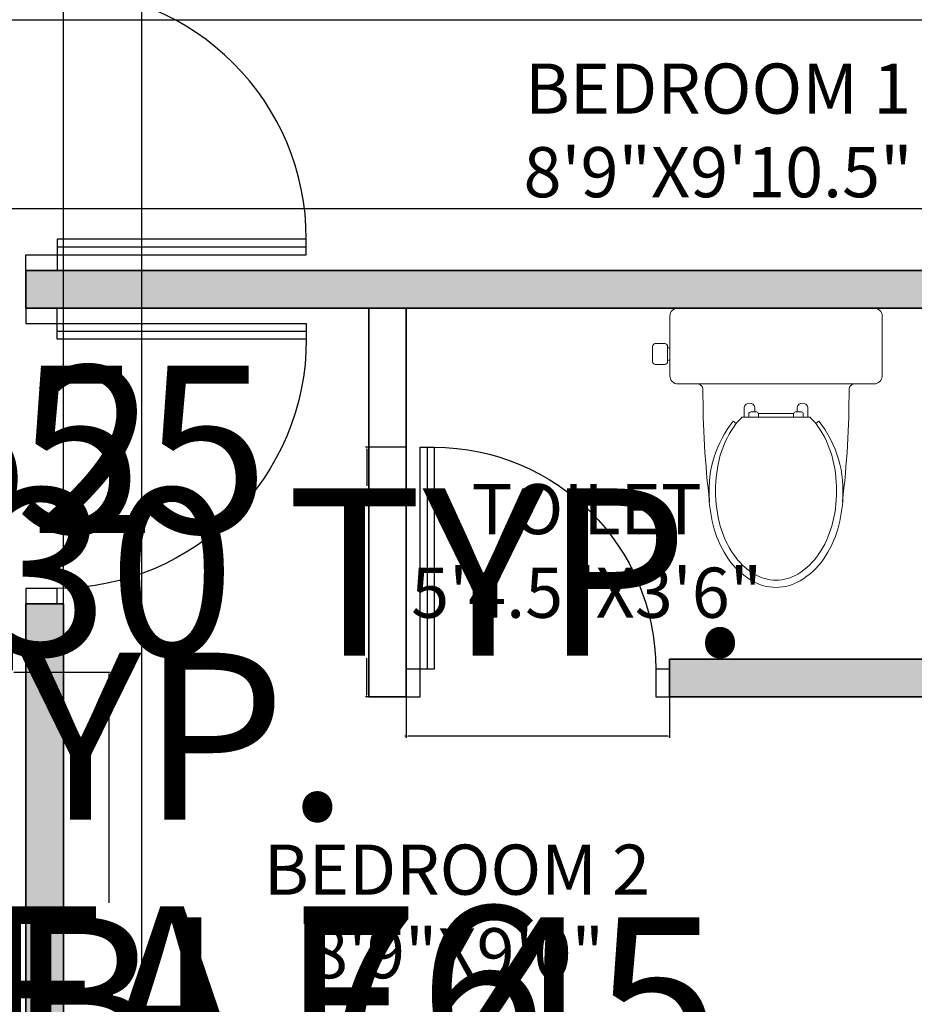
# Model space of a CAD drawing. Units: inches. Extents: x 305 to 776, y 38 to 479.
# Tile 12 of 14: x 511 to 618, y 214 to 332. Entities that reach past the tile are written whole.
import ezdxf

# ---------------------------------------------------------------- set-up
doc = ezdxf.new("R2010")
doc.units = ezdxf.units.IN
doc.header["$MEASUREMENT"] = 0
for name, color, linetype, lineweight in [('A-ANNO-DIMS', 2, 'Continuous', 18), ('A-AREA-IDEN', 7, 'Continuous', 18), ('A-DOOR', 4, 'Continuous', 25), ('A-FLOR-FIXT', 9, 'Continuous', 18), ('A-WALL', 7, 'Continuous', 35), ('A-WALL-PATT', 252, 'Continuous', 13)]:
    doc.layers.add(name, color=color, linetype=linetype, lineweight=lineweight)
doc.styles.get("Standard").update_dxf_attribs({"font": 'arial.ttf'})
doc.dimstyles.get("Standard").update_dxf_attribs({"dimtxt": 20, "dimasz": 0.18, "dimexe": 0.18, "dimexo": 0.0625, "dimgap": 0.09, "dimtad": 0, "dimtih": 1, "dimtoh": 1, "dimdec": 4, "dimzin": 0, "dimdsep": 46, "dimtxsty": 'Standard', "dimcen": 0.09, "dimadec": 0, "dimazin": 0, "dimtfac": 1, "dimtdec": 4, "dimtofl": 0, "dimtmove": 0, "dimatfit": 3, "dimfxl": 1, "dimtolj": 1, "dimtzin": 0, "dimarcsym": 0})

# ---------------------------------------------------------------- blocks, each defined once
blk = doc.blocks.new('A$C296830DC')
blk.add_line((828.9, 852.6), (828.9, 94.7))
for points in [[(852.6, 94.7), (852.6, 852.6), (805.3, 852.6), (805.3, 94.7)], [(47.4, 94.7), (47.4, 0), (0, 0), (0, 94.7)], [(900, 94.7), (900, 0), (852.6, 0), (852.6, 94.7)]]:
    blk.add_lwpolyline(points, close=True)
blk.add_arc((805.3, 94.7), 757.9, 90, 180)
blk = doc.blocks.new('t')
for points in [[(1220.28, 636.63), (1208.55, 636.63, 0.414214), (1207.58, 635.67), (1207.58, 631.86, 0.414214)], [(1220.28, 636.63), (1232.02, 636.63, -0.414214), (1232.98, 635.67), (1232.98, 628.51, -0.414214), (1232.02, 627.55), (1229.53, 627.55)], [(1207.31, 631.86), (1207.31, 632.04, 0.414214), (1206.99, 632.37), (1205.84, 632.37, 0.414214), (1205.52, 632.04), (1205.52, 630.21, 0.414214), (1205.84, 629.89)], [(1207.31, 630.39), (1207.31, 631.86, 0.414214)], [(1207.58, 631.86), (1207.58, 630.39, 0.414214)], [(1205.84, 629.89), (1206.99, 629.89, 0.414214), (1207.31, 630.21), (1207.31, 630.39, 0.414214)], [(1207.58, 630.39), (1207.58, 628.51, 0.414214), (1208.55, 627.55), (1211.03, 627.55)], [(1211.03, 627.55, -0.279901), (1211.54, 626.96, 0.030761), (1212.34, 613.45, 16.522544)], [(1229.53, 627.55, 0.279901), (1229.02, 626.96, -0.030761), (1228.22, 613.45, -16.522544)], [(1216.48, 623.56), (1216.48, 624.75, -0.788198), (1217.76, 624.75), (1217.76, 624.2)], [(1224.09, 623.56), (1224.09, 624.75, 0.788198), (1222.8, 624.75), (1222.8, 624.2)], [(1213.04, 614.76, 0.068564), (1213.62, 610.52, 0.080689), (1215.16, 607.21, 0.107047), (1217.67, 604.81, 0.137952), (1220.28, 604.08, 0.137952), (1222.89, 604.81, 0.107047), (1225.4, 607.21, 0.080689), (1226.94, 610.52, 0.068564), (1227.53, 614.76, 0.068564), (1226.94, 619.01, 0.080689), (1225.4, 622.31, 0.049741), (1224.36, 623.56, 0.137952)], [(1216.2, 623.56, 0.049741), (1215.16, 622.31, 0.080689), (1213.62, 619.01, 0.068564), (1213.04, 614.76, 0.068564)], [(1217.03, 623.56), (1217.03, 623.98, -0.414214), (1217.26, 624.2), (1217.94, 624.2, -0.414214), (1218.17, 623.98), (1218.17, 623.56)], [(1223.54, 623.56), (1223.54, 623.98, 0.414214), (1223.31, 624.2), (1222.62, 624.2, 0.414214), (1222.39, 623.98), (1222.39, 623.56)], [(1212.3, 614.03, -0.186192), (1215.17, 623.1), (1215.53, 622.81)], [(1228.22, 613.45, 0.197511), (1225.39, 623.1), (1225.04, 622.81)], [(1212.27, 614.03, 0.059006), (1212.9, 610.18, 0.081908), (1214.61, 606.59, 0.106902), (1217.38, 604.01, 0.135271), (1220.28, 603.21, 0.135271)], [(1212.34, 613.45, -0.010918), (1212.3, 614.03)], [(1220.28, 603.21, 0.135271), (1223.19, 604.01, 0.106902), (1225.95, 606.59, 0.081908), (1227.66, 610.18, 0.059006), (1228.29, 614.03, 0.070136)]]:
    blk.add_lwpolyline(points, format="xyb")
for points in [[(1207.31, 631.86), (1207.58, 631.86)], [(1207.31, 630.39), (1207.58, 630.39)], [(1211.03, 627.55), (1220.28, 627.55)], [(1229.53, 627.55), (1220.28, 627.55)], [(1216.2, 623.56), (1224.36, 623.56)], [(1218.17, 624.02), (1222.39, 624.02)]]:
    blk.add_lwpolyline(points)
blk = doc.blocks.new('*D19')
at = {"layer": 'A-ANNO-DIMS', "color": 0, "lineweight": -2, "transparency": 16777216}
for p, q in [((557.63, 250.82), (557.63, 245.98)), ((589.13, 250.82), (589.13, 245.98)), ((557.63, 246.16), (557.45, 246.16)), ((588.95, 246.16), (557.81, 246.16))]:
    blk.add_line(p, q, dxfattribs=at)
at = {"layer": 'A-ANNO-DIMS', "color": 0, "transparency": 16777216}
for points in [[(557.81, 246.19), (557.81, 246.13), (557.63, 246.16)], [(588.95, 246.19), (588.95, 246.13), (589.13, 246.16)]]:
    blk.add_solid(points, dxfattribs=at)
at = {"layer": 'Defpoints', "color": 0, "transparency": 16777216}
for p in [(557.63, 250.88), (589.13, 250.88), (557.63, 246.16)]:
    blk.add_point(p, dxfattribs=at)
at = {"layer": 'A-ANNO-DIMS', "color": 0, "transparency": 16777216, "insert": (463.39, 246.16), "char_height": 20, "attachment_point": 5}
blk.add_mtext('\\A1;DOOR 32 TYP.', dxfattribs=at)
blk = doc.blocks.new('*D20')
at = {"layer": 'A-ANNO-DIMS', "color": 0, "lineweight": -2, "transparency": 16777216}
for p, q in [((557.57, 280.72), (552.73, 280.72)), ((552.91, 280.54), (552.91, 276.11)), ((552.91, 251.06), (552.91, 255.49)), ((557.57, 250.88), (552.73, 250.88))]:
    blk.add_line(p, q, dxfattribs=at)
at = {"layer": 'A-ANNO-DIMS', "color": 0, "transparency": 16777216}
for points in [[(552.88, 280.54), (552.94, 280.54), (552.91, 280.72)], [(552.88, 251.06), (552.94, 251.06), (552.91, 250.88)]]:
    blk.add_solid(points, dxfattribs=at)
at = {"layer": 'Defpoints', "color": 0, "transparency": 16777216}
for p in [(552.91, 280.72), (557.63, 280.72), (557.63, 250.88)]:
    blk.add_point(p, dxfattribs=at)
at = {"layer": 'A-ANNO-DIMS', "color": 0, "transparency": 16777216, "insert": (552.91, 265.8), "char_height": 20, "attachment_point": 5}
blk.add_mtext('\\A1;30 TYP.', dxfattribs=at)
blk = doc.blocks.new('*D27')
at = {"layer": 'A-ANNO-DIMS', "color": 0, "lineweight": -2, "transparency": 16777216}
for p, q in [((630.7, 388.18), (639.63, 388.18)), ((639.45, 388), (639.45, 369.09)), ((639.45, 329.56), (639.45, 348.47)), ((630.7, 329.38), (639.63, 329.38))]:
    blk.add_line(p, q, dxfattribs=at)
at = {"layer": 'A-ANNO-DIMS', "color": 0, "transparency": 16777216}
for points in [[(639.42, 388), (639.48, 388), (639.45, 388.18)], [(639.42, 329.56), (639.48, 329.56), (639.45, 329.38)]]:
    blk.add_solid(points, dxfattribs=at)
at = {"layer": 'Defpoints', "color": 0, "transparency": 16777216}
for p in [(630.63, 388.18), (630.63, 329.38), (639.45, 329.38)]:
    blk.add_point(p, dxfattribs=at)
at = {"layer": 'A-ANNO-DIMS', "color": 0, "transparency": 16777216, "insert": (639.45, 358.78), "char_height": 20, "attachment_point": 5}
blk.add_mtext('\\A1;W3 59 TYP.', dxfattribs=at)
blk = doc.blocks.new('*D33')
at = {"layer": 'A-ANNO-DIMS', "color": 0, "lineweight": -2, "transparency": 16777216}
for p, q in [((440.93, 307.95), (449.29, 307.95)), ((449.11, 307.77), (449.11, 290.9)), ((449.11, 253.16), (449.11, 270.03)), ((440.93, 252.98), (449.29, 252.98))]:
    blk.add_line(p, q, dxfattribs=at)
at = {"layer": 'A-ANNO-DIMS', "color": 0, "transparency": 16777216}
for points in [[(449.08, 307.77), (449.14, 307.77), (449.11, 307.95)], [(449.08, 253.16), (449.14, 253.16), (449.11, 252.98)]]:
    blk.add_solid(points, dxfattribs=at)
at = {"layer": 'Defpoints', "color": 0, "transparency": 16777216}
for p in [(440.86, 307.95), (449.11, 307.95), (440.86, 252.98)]:
    blk.add_point(p, dxfattribs=at)
at = {"layer": 'A-ANNO-DIMS', "color": 0, "transparency": 16777216, "insert": (449.11, 280.47), "char_height": 20, "attachment_point": 5}
blk.add_mtext('\\A1;DINING SET 55', dxfattribs=at)
blk = doc.blocks.new('*D35')
at = {"layer": 'A-ANNO-DIMS', "color": 0, "lineweight": -2, "transparency": 16777216}
for p, q in [((510.7, 253.8), (522.21, 253.8)), ((522.03, 253.62), (522.03, 226.23)), ((522.03, 177.97), (522.03, 205.36)), ((510.7, 177.79), (522.21, 177.79))]:
    blk.add_line(p, q, dxfattribs=at)
at = {"layer": 'A-ANNO-DIMS', "color": 0, "transparency": 16777216}
for points in [[(522, 253.62), (522.06, 253.62), (522.03, 253.8)], [(522, 177.97), (522.06, 177.97), (522.03, 177.79)]]:
    blk.add_solid(points, dxfattribs=at)
at = {"layer": 'Defpoints', "color": 0, "transparency": 16777216}
for p in [(510.63, 253.8), (522.03, 253.8), (510.63, 177.79)]:
    blk.add_point(p, dxfattribs=at)
at = {"layer": 'A-ANNO-DIMS', "color": 0, "transparency": 16777216, "insert": (522.03, 215.8), "char_height": 20, "attachment_point": 5}
blk.add_mtext('\\A1;SOFA 76', dxfattribs=at)
blk = doc.blocks.new('*D37')
at = {"layer": 'A-ANNO-DIMS', "color": 0, "lineweight": -2, "transparency": 16777216}
for p, q in [((476.35, 237.03), (483.22, 237.03)), ((483.04, 236.85), (483.04, 224.94)), ((483.04, 192.15), (483.04, 204.06)), ((476.35, 191.97), (483.22, 191.97))]:
    blk.add_line(p, q, dxfattribs=at)
at = {"layer": 'A-ANNO-DIMS', "color": 0, "transparency": 16777216}
for points in [[(483.01, 236.85), (483.07, 236.85), (483.04, 237.03)], [(483.01, 192.15), (483.07, 192.15), (483.04, 191.97)]]:
    blk.add_solid(points, dxfattribs=at)
at = {"layer": 'Defpoints', "color": 0, "transparency": 16777216}
for p in [(476.28, 237.03), (483.04, 237.03), (476.28, 191.97)]:
    blk.add_point(p, dxfattribs=at)
at = {"layer": 'A-ANNO-DIMS', "color": 0, "transparency": 16777216, "insert": (483.04, 214.5), "char_height": 20, "attachment_point": 5}
blk.add_mtext('\\A1;COFFEE TABLE 45', dxfattribs=at)
blk = doc.blocks.new('*D49')
at = {"layer": 'A-ANNO-DIMS', "color": 0, "lineweight": -2, "transparency": 16777216}
for p, q in [((399.7, 331.88), (648.81, 331.88)), ((648.63, 331.7), (648.63, 330.88)), ((648.63, 309.46), (648.63, 310.28)), ((399.7, 309.28), (648.81, 309.28))]:
    blk.add_line(p, q, dxfattribs=at)
at = {"layer": 'A-ANNO-DIMS', "color": 0, "transparency": 16777216}
for points in [[(648.6, 331.7), (648.66, 331.7), (648.63, 331.88)], [(648.6, 309.46), (648.66, 309.46), (648.63, 309.28)]]:
    blk.add_solid(points, dxfattribs=at)
at = {"layer": 'Defpoints', "color": 0, "transparency": 16777216}
for p in [(399.63, 331.88), (648.63, 331.88), (399.63, 309.28)]:
    blk.add_point(p, dxfattribs=at)
at = {"layer": 'A-ANNO-DIMS', "color": 0, "transparency": 16777216, "insert": (648.63, 320.58), "char_height": 20, "attachment_point": 5}
blk.add_mtext('\\A1;22.6', dxfattribs=at)
blk = doc.blocks.new('*D58')
at = {"layer": 'A-ANNO-DIMS', "color": 0, "lineweight": -2, "transparency": 16777216}
for p, q in [((516.63, 138.44), (516.63, 447.56)), ((516.81, 447.38), (525.83, 447.38)), ((526.01, 138.44), (526.01, 447.56)), ((526.01, 447.38), (526.19, 447.38))]:
    blk.add_line(p, q, dxfattribs=at)
at = {"layer": 'A-ANNO-DIMS', "color": 0, "transparency": 16777216}
for points in [[(516.81, 447.41), (516.81, 447.35), (516.63, 447.38)], [(525.83, 447.41), (525.83, 447.35), (526.01, 447.38)]]:
    blk.add_solid(points, dxfattribs=at)
at = {"layer": 'Defpoints', "color": 0, "transparency": 16777216}
for p in [(526.01, 447.38), (516.63, 138.38), (526.01, 138.38)]:
    blk.add_point(p, dxfattribs=at)
at = {"layer": 'A-ANNO-DIMS', "color": 0, "transparency": 16777216, "insert": (560.1, 447.38), "char_height": 20, "attachment_point": 5}
blk.add_mtext('\\A1;9.375', dxfattribs=at)
blk = doc.blocks.new('*D60')
at = {"layer": 'A-ANNO-DIMS', "color": 0, "lineweight": -2, "transparency": 16777216}
for p, q in [((428.26, 331.82), (428.26, 51.2)), ((465.63, 331.82), (465.63, 51.2)), ((428.44, 51.38), (465.45, 51.38)), ((465.63, 51.38), (465.81, 51.38))]:
    blk.add_line(p, q, dxfattribs=at)
at = {"layer": 'A-ANNO-DIMS', "color": 0, "transparency": 16777216}
for points in [[(428.44, 51.41), (428.44, 51.35), (428.26, 51.38)], [(465.45, 51.41), (465.45, 51.35), (465.63, 51.38)]]:
    blk.add_solid(points, dxfattribs=at)
at = {"layer": 'Defpoints', "color": 0, "transparency": 16777216}
for p in [(428.26, 331.88), (465.63, 331.88), (465.63, 51.38)]:
    blk.add_point(p, dxfattribs=at)
at = {"layer": 'A-ANNO-DIMS', "color": 0, "transparency": 16777216, "insert": (499.64, 51.38), "char_height": 20, "attachment_point": 5}
blk.add_mtext('\\A1;37.37', dxfattribs=at)
blk = doc.blocks.new('*D61')
at = {"layer": 'A-ANNO-DIMS', "color": 0, "lineweight": -2, "transparency": 16777216}
for p, q in [((437.73, 398.69), (437.73, 51.2)), ((465.63, 398.69), (465.63, 51.2)), ((437.91, 51.38), (465.45, 51.38)), ((465.63, 51.38), (465.81, 51.38))]:
    blk.add_line(p, q, dxfattribs=at)
at = {"layer": 'A-ANNO-DIMS', "color": 0, "transparency": 16777216}
for points in [[(437.91, 51.41), (437.91, 51.35), (437.73, 51.38)], [(465.45, 51.41), (465.45, 51.35), (465.63, 51.38)]]:
    blk.add_solid(points, dxfattribs=at)
at = {"layer": 'Defpoints', "color": 0, "transparency": 16777216}
for p in [(437.73, 398.75), (465.63, 398.75), (465.63, 51.38)]:
    blk.add_point(p, dxfattribs=at)
at = {"layer": 'A-ANNO-DIMS', "color": 0, "transparency": 16777216, "insert": (492.07, 51.38), "char_height": 20, "attachment_point": 5}
blk.add_mtext('\\A1;27.9', dxfattribs=at)
blk = doc.blocks.new('*D75')
at = {"layer": 'A-ANNO-DIMS', "color": 0, "lineweight": -2, "transparency": 16777216}
for p, q in [((413.29, 280.47), (413.47, 280.47)), ((413.38, 280.38), (413.38, 280.56)), ((435.4, 280.46), (427.32, 280.46))]:
    blk.add_line(p, q, dxfattribs=at)
at = {"layer": 'A-ANNO-DIMS', "color": 0, "transparency": 16777216}
blk.add_solid([(427.32, 280.49), (427.32, 280.43), (427.14, 280.46)], dxfattribs=at)
at = {"layer": 'Defpoints', "color": 0, "transparency": 16777216}
for p in [(399.62, 280.47), (427.14, 280.46)]:
    blk.add_point(p, dxfattribs=at)
at = {"layer": 'A-ANNO-DIMS', "color": 0, "transparency": 16777216, "insert": (480.01, 280.46), "char_height": 20, "attachment_point": 5}
blk.add_mtext('\\A1;∅27.52', dxfattribs=at)

msp = doc.modelspace()

# ---------------------------------------------------------------- hatches: boundary and pattern name
at = {"layer": 'A-WALL-PATT'}
h = msp.add_hatch(color=256, dxfattribs=at)
h.dxf.hatch_style = 1
h.paths.add_polyline_path([(481.3329, 429.382), (390.6329, 429.382), (390.6329, 398.067), (399.6329, 398.067), (399.6329, 420.382), (465.6329, 420.382), (465.6329, 331.882), (470.1329, 331.882), (470.1329, 355.882), (512.1329, 355.882), (512.1329, 337.282), (512.1329, 337.282), (515.8592, 337.282), (516.6329, 337.282), (516.6329, 360.382), (513.3171, 360.382), (470.1329, 360.382), (470.1329, 420.382), (481.3329, 420.382)])
h.paths.add_polyline_path([(630.6329, 429.382), (500.9329, 429.382), (500.9329, 420.382), (502.8693, 420.382), (512.1329, 420.382), (512.1329, 391.882), (516.6329, 391.882), (516.6329, 420.382), (621.6329, 420.382), (621.6329, 388.182), (630.6329, 388.182)])
h.paths.add_polyline_path([(630.6329, 329.382), (621.6329, 329.382), (621.6329, 301.882), (512.1329, 301.882), (512.1329, 297.382), (515.8592, 297.382), (557.6329, 297.382), (621.6329, 297.382), (621.6329, 286.182), (630.6329, 286.182)])
h.paths.add_polyline_path([(630.6329, 266.582), (621.6329, 266.582), (621.6329, 255.382), (589.1329, 255.382), (589.1329, 250.882), (621.6329, 250.882), (621.6329, 226.282), (630.6329, 226.282)])
h.paths.add_polyline_path([(630.6329, 167.482), (621.6329, 167.482), (621.6329, 149.1444), (621.6329, 142.882), (516.6329, 142.882), (516.6329, 261.982), (512.1329, 261.982), (512.1329, 138.382), (621.6329, 138.382), (621.6329, 78.382), (512.1329, 78.382), (512.1329, 69.382), (630.6329, 69.382)])
h.paths.add_polyline_path([(464.1329, 138.382), (476.7329, 138.382), (476.7329, 142.1084), (476.7329, 142.882), (459.6329, 142.882), (459.6329, 78.382), (399.6329, 78.382), (399.6329, 98.582), (390.6329, 98.582), (390.6329, 69.382), (464.1329, 69.382)])
h.paths.add_polyline_path([(459.6329, 142.882), (439.3329, 142.882), (439.3329, 138.382), (459.6329, 138.382)], flags=17)
h.paths.add_polyline_path([(399.6329, 138.382), (403.9329, 138.382), (403.9329, 141.5545), (403.9329, 141.5545), (403.9329, 142.882), (399.6329, 142.882), (399.6329, 250.4819), (390.6329, 250.4819), (390.6329, 118.182), (399.6329, 118.182)])
h.paths.add_polyline_path([(399.6329, 331.882), (428.2629, 331.882), (428.2629, 336.382), (399.6329, 336.382), (399.6329, 358.697), (390.6329, 358.697), (390.6329, 309.2819), (399.6329, 309.2819)])

# ---------------------------------------------------------------- linework, layer by layer
at = {"layer": 'A-WALL'}
for p, q in [((621.6329, 301.882), (512.1329, 301.882)), ((512.1329, 301.882), (512.1329, 297.382)), ((557.6329, 297.382), (512.1329, 297.382)), ((553.1329, 250.882), (553.1329, 297.382)), ((621.6329, 297.382), (557.6329, 297.382)), ((557.6329, 250.882), (557.6329, 297.382)), ((621.6329, 297.382), (557.6329, 297.382)), ((516.6329, 261.982), (512.1329, 261.982)), ((512.1329, 261.982), (512.1329, 138.382)), ((516.6329, 261.982), (516.6329, 142.882)), ((621.6329, 255.382), (589.1329, 255.382)), ((589.1329, 250.882), (589.1329, 255.382)), ((557.6329, 250.882), (553.1329, 250.882)), ((621.6329, 250.882), (589.1329, 250.882))]:
    msp.add_line(p, q, dxfattribs=at)

# ---------------------------------------------------------------- block references
at = {"layer": 'A-DOOR', "yscale": 0.0393333333333333, "zscale": 0.0393333333333333, "rotation": 270}
for p, xscale in [((512.1329, 337.282), 0.0393333333333333), ((512.1329, 261.982), -0.0393333333333333)]:
    msp.add_blockref('A$C296830DC', p, dxfattribs=dict(at, xscale=xscale))
at = {"layer": 'A-DOOR', "xscale": -0.035, "yscale": 0.035, "zscale": 0.035}
msp.add_blockref('A$C296830DC', (589.1329, 250.882), dxfattribs=at)
at = {"layer": 'A-FLOR-FIXT'}
msp.add_blockref('t', (-618.4252, -339.2468), dxfattribs=at)

# ---------------------------------------------------------------- texts
at = {"layer": 'A-AREA-IDEN', "char_height": 6, "attachment_point": 1}
for s, insert in [('\\pxqc;BEDROOM 1\\P8\'9"X9\'10.5"', (555.828, 326.6395)), ('\\pxqc;TOILET\\P5\'4.5"X3\'6"', (540.1156, 276.3267)), ('\\pxqc;BEDROOM 2\\P8\'9"X9\'0"', (524.599, 233.1913))]:
    msp.add_mtext_dynamic_manual_height_columns(s, width=78.185, gutter_width=1, heights=[0], dxfattribs=dict(at, insert=insert))

# ---------------------------------------------------------------- dimensions: what is measured, and where the dimension line sits
at = {"layer": 'A-ANNO-DIMS'}
for base, p1, p2, override, picture, middle in [((526.0079, 447.3835), (516.6329, 138.382), (526.0079, 138.382), {"dimdec": 3, "dimlfac": 1, "dimrnd": 0, "dimzin": 0, "dimdsep": 46, "dimlunit": 2}, '*D58', (560.0978, 447.3835)), ((465.6329, 51.3805), (437.7303, 398.7487), (465.6329, 398.7487), {"dimdec": 1, "dimlfac": 1, "dimrnd": 0, "dimzin": 0, "dimdsep": 46, "dimlunit": 2}, '*D61', (492.0693, 51.3805)), ((465.6329, 51.3805), (428.2629, 331.882), (465.6329, 331.882), {"dimdec": 2, "dimlfac": 1, "dimrnd": 0, "dimzin": 0, "dimdsep": 46, "dimlunit": 2}, '*D60', (499.641, 51.3805))]:
    dim = msp.add_linear_dim(base=base, p1=p1, p2=p2, dimstyle='Standard', override=override, dxfattribs=at)
    dim.commit()
    dim.dimension.update_dxf_attribs({"geometry": picture, "text_midpoint": middle})
for base, p1, p2, angle, text, picture, middle in [((639.4529, 329.382), (630.6329, 388.182), (630.6329, 329.382), 270, 'W3 <> TYP.', '*D27', (639.4529, 358.782)), ((449.1096, 307.9493), (440.8644, 252.9815), (440.8644, 307.9493), 90, 'DINING SET <>', '*D33', (449.1096, 280.4654)), ((552.9079, 280.7241), (557.6329, 250.882), (557.6329, 280.7241), 90, '<> TYP.', '*D20', (552.9079, 265.8031)), ((557.6329062952, 246.15704135), (589.1329062952, 250.88204135), (557.6329062952, 250.88204135), 180, 'DOOR <> TYP.', '*D19', (463.3929199378, 246.15704135)), ((483.0416, 237.0288), (476.2832, 191.9726), (476.2832, 237.0288), 90, 'COFFEE TABLE <>', '*D37', (483.0416, 214.5007)), ((522.0346, 253.8016), (510.6329, 177.7903), (510.6329, 253.8016), 90, 'SOFA <>', '*D35', (522.0346, 215.796))]:
    dim = msp.add_linear_dim(base=base, p1=p1, p2=p2, angle=angle, text=text, dimstyle='Standard', override={"dimdec": 0, "dimlfac": 1, "dimrnd": 0, "dimzin": 0, "dimdsep": 46, "dimlunit": 2}, dxfattribs=at)
    dim.commit()
    dim.dimension.update_dxf_attribs({"geometry": picture, "text_midpoint": middle})
dim = msp.add_linear_dim(base=(648.6344, 331.882), p1=(399.6329, 309.2819), p2=(399.6329, 331.882), angle=90, dimstyle='Standard', override={"dimdec": 1, "dimlfac": 1, "dimrnd": 0, "dimzin": 0, "dimdsep": 46, "dimlunit": 2}, dxfattribs=at)
dim.commit()
dim.dimension.update_dxf_attribs({"geometry": '*D49', "text_midpoint": (648.6344, 320.582)})
dim = msp.add_diameter_dim_2p(p1=(399.6205, 280.4658), p2=(427.1405, 280.465), dimstyle='Standard', override={"dimdec": 2, "dimlfac": 1, "dimrnd": 0, "dimzin": 0, "dimdsep": 46, "dimlunit": 2}, dxfattribs=at)
dim.commit()
dim.dimension.update_dxf_attribs({"geometry": '*D75', "text_midpoint": (435.3965, 280.4648), "dimtype": 163})

doc.saveas('drawing.dxf')
